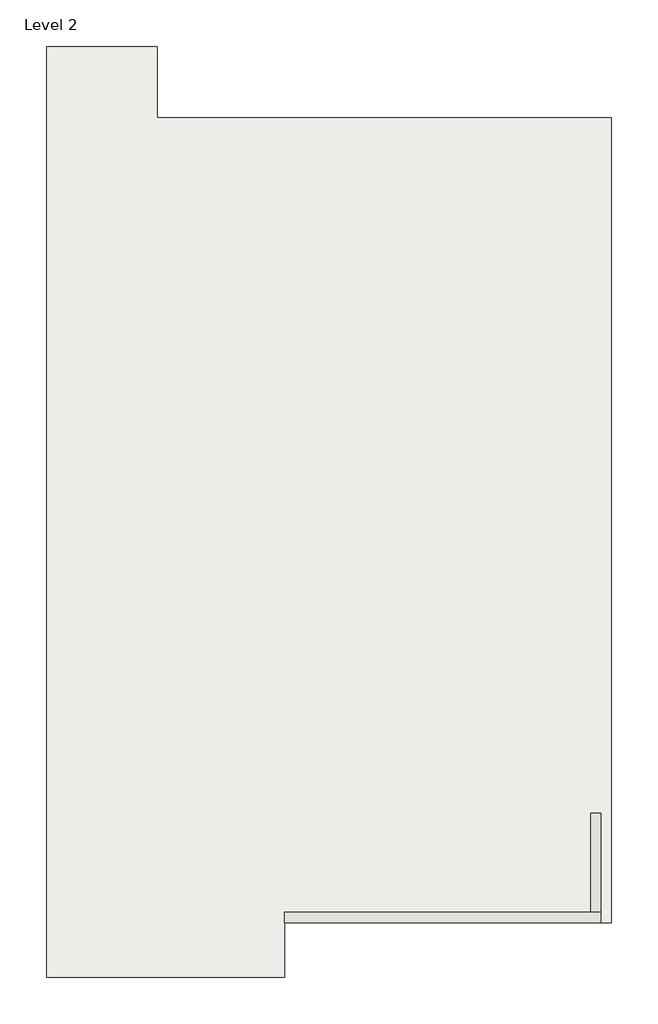
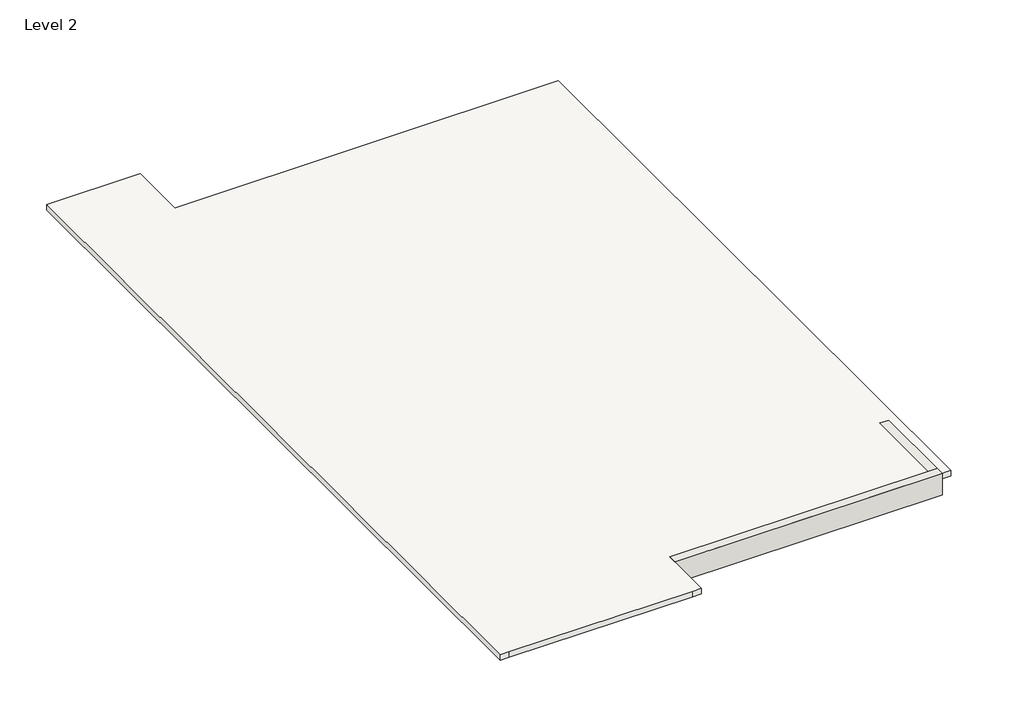
# One storey: 2 walls, 1 roof.
"""IFC4 building model written with IfcOpenShell, lengths in millimetres."""

from ifc_helpers import new_model, si_unit, frame, origin, place, context, project, spatial, polyline, outline, extrude, faceted_brep, element, save

model = new_model("IFC4")

# Units and contexts
model_context = context("Model", 3, world=origin())
ifc_project = project(units=[si_unit("LENGTHUNIT", "METRE", prefix="MILLI")], contexts=[model_context])

# Site, building, storey
site = spatial("IfcSite", under=ifc_project)
building = spatial("IfcBuilding", under=site)
storey = spatial("IfcBuildingStorey", under=building, Name="Level 2", Elevation=3657.6)

# Roof
placement = place(None, origin())
element("IfcRoof", 1, ObjectType="Generic - 12\"", at=placement, inside=storey, context=model_context, shape_type="SweptSolid", body=[
    extrude(outline(polyline([(-5476.8909398, -6555.6648025), (-10315.5909398, -6555.6648025), (-10544.1909398, -6555.6648025), (-10544.1909398, 14151.9493277), (-8080.9689749, 14151.9493277), (-8080.9689749, 12570.5351975), (2028.8090602, 12570.5351975), (2028.8090602, -5336.4648025), (-5248.2909398, -5336.4648025), (-5248.2909398, -6555.6648025), (-5476.8909398, -6555.6648025)])), frame((0.0, 0.0, 3657.6), z_axis=(0.0, 0.0, 1.0), x_axis=(1.0, 0.0, 0.0)), (0.0, 0.0, 1.0), 152.4),
])

# Walls
element("IfcWall", 2, ObjectType="9\" wall", at=placement, inside=storey, context=model_context, shape_type="Brep", body=[
    faceted_brep([(-5248.2909398, -5336.4648025, 3209.3762568), (1800.2090602, -5336.4648025, 3209.3762568), (1800.2090602, -5336.4648025, 3810.0), (-5248.2909398, -5336.4648025, 3810.0), (-5248.2909398, -5107.8648025, 3209.3762568), (-5248.2909398, -5107.8648025, 3810.0), (1571.6090602, -5107.8648025, 3810.0), (1800.2090602, -5107.8648025, 3810.0), (1800.2090602, -5107.8648025, 3260.1762568), (1800.2090602, -5107.8648025, 3209.3762568)], [[[0, 1, 2, 3]], [[4, 5, 6, 7, 8, 9]], [[1, 0, 4, 9]], [[3, 2, 7, 6, 5]], [[2, 1, 9, 8, 7]], [[0, 3, 5, 4]]]),
])
element("IfcWall", 3, ObjectType="9\" wall", at=placement, inside=storey, context=model_context, shape_type="Brep", body=[
    faceted_brep([(1800.2090602, -5107.8648025, 3260.1762568), (1800.2090602, -2898.0648025, 3260.1762568), (1800.2090602, -2898.0648025, 3657.6), (1800.2090602, -2898.0648025, 3810.0), (1800.2090602, -5107.8648025, 3810.0), (1571.6090602, -5107.8648025, 3260.1762568), (1571.6090602, -5107.8648025, 3810.0), (1571.6090602, -2898.0648025, 3810.0), (1571.6090602, -2898.0648025, 3260.1762568)], [[[0, 1, 2, 3, 4]], [[5, 6, 7, 8]], [[1, 0, 5, 8]], [[4, 3, 7, 6]], [[0, 4, 6, 5]], [[3, 2, 1, 8, 7]]]),
])

save(model, "model.ifc")

# Revit data of these elements
# Type "Generic - 12\""
#   Assembly Code = "B1020"
#   Layers, outside or top first: 0' - 6" "Laminate, Ivory, Matte" (function 1)
# Type "9\" wall"
#   Assembly Code = "B2010"
#   Layers, outside or top first: 0' - 9" "Laminate, Ivory, Matte" (function 1)
# Element 1 (IfcRoof, "Generic - 12\"")
#   built-in parameter 1001705 = 12.5 (stored number, unit not read)
#   built-in parameter 1001710 = 33615
#   Phase Created = New Construction
#   Materials on its faces: "Laminate, Ivory, Matte"
# Element 2 (IfcWall, "9\" wall")
#   built-in parameter 1001111 = -1' - 5.6466"
#   Top Offset = 0' - 0"
#   Base Offset = -1' - 5.6466"
#   wall height = 1' - 11.6466"
#   Phase Created = New Construction
#   Base Constraint = Level 2
#   Top Constraint = Level 3
#   Materials on its faces: "Laminate, Ivory, Matte"
# Element 3 (IfcWall, "9\" wall")
#   built-in parameter 1001111 = -1' - 3.6466"
#   Top Offset = 0' - 0"
#   Base Offset = -1' - 3.6466"
#   wall height = 1' - 9.6466"
#   Phase Created = New Construction
#   Base Constraint = Level 2
#   Top Constraint = Level 3
#   Materials on its faces: "Laminate, Ivory, Matte"
# Materials
#   "Laminate, Ivory, Matte": class "Plastic", colour RGB 247 247 239, transparency 0, Description = "Plastic Laminate - Ivory, Matte", Cost = 0
